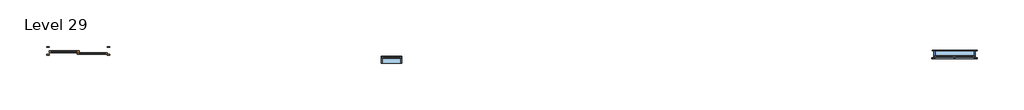
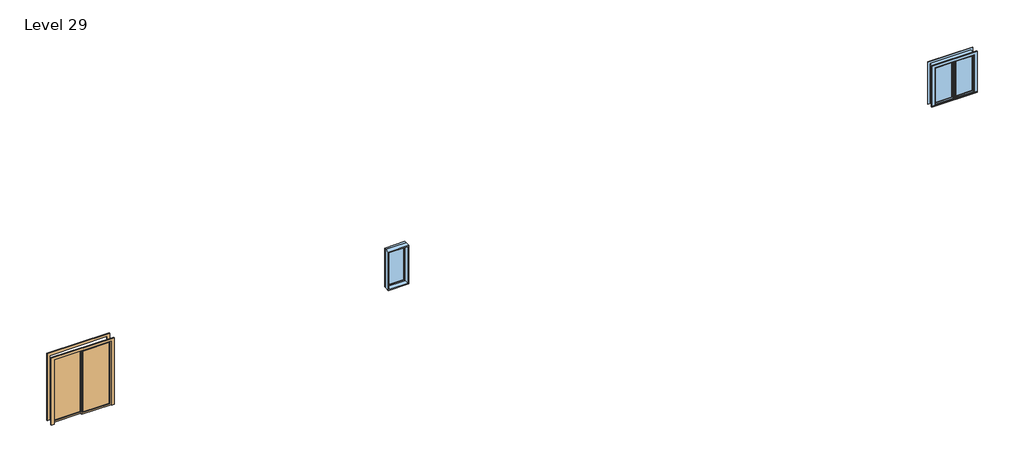
# One storey: 2 windows, 1 door.
"""IFC4 building model written with IfcOpenShell, lengths in millimetres."""

from ifc_helpers import new_model, si_unit, origin, place, context, project, spatial, transform, mapped, element, save
from components import door_076b30e0, window_0862ab64, window_80bd9af0

model = new_model("IFC4")

# Units and contexts
model_context = context("Model", 3, world=origin())
ifc_project = project(units=[si_unit("LENGTHUNIT", "METRE", prefix="MILLI")], contexts=[model_context])

# Site, building, storey
site = spatial("IfcSite", under=ifc_project)
building = spatial("IfcBuilding", under=site)
storey = spatial("IfcBuildingStorey", under=building, Name="Level 29", Elevation=49682.4)

# Door
placement = place(None, origin())
door_shape = door_076b30e0(model_context)
element("IfcDoor", 1, ObjectType="Door-Double-Sliding : 68\" x 80\"", at=placement, inside=storey, context=model_context, shape_type="MappedRepresentation", body=[
    mapped(door_shape, transform((-16064.585279, -12227.7237084, 49682.4), x_axis=(-1.0, 0.0, 0.0), y_axis=(0.0, -1.0, 0.0), z_axis=(0.0, 0.0, 1.0))),
])

# Windows
window_shape = window_0862ab64(model_context)
element("IfcWindow", 2, ObjectType="Casement Dbl with Trim : 48\" x 48\"", at=placement, inside=storey, context=model_context, shape_type="MappedRepresentation", body=[
    mapped(window_shape, transform((9924.3594464, -12437.2737084, 49682.4), x_axis=(-1.0, 0.0, 0.0), y_axis=(0.0, -1.0, 0.0), z_axis=(0.0, 0.0, 1.0))),
])
window_2_shape = window_80bd9af0(model_context)
element("IfcWindow", 3, ObjectType="Fixed : 24\" x 48\"", at=placement, inside=storey, context=model_context, shape_type="MappedRepresentation", body=[
    mapped(window_2_shape, transform((-6730.085279, -12617.2007309, 49682.4), x_axis=(1.0, 0.0, 0.0), y_axis=(0.0, 1.0, 0.0), z_axis=(0.0, 0.0, 1.0))),
])

save(model, "model.ifc")

# Revit data of these elements
# Type "Door-Double-Sliding : 68\" x 80\""
#   Type Mark = "10"
#   Construction Type Id = "opn-d45"
#   Assembly Code = "C1020"
#   Analytic Construction = "Wood frame, double glass door "
#   Thickness = 0' - 2"
#   Thermal Resistance (R) = 1.8150 (h·ft²·°F)/BTU
#   Heat Transfer Coefficient (U) = 0.5510 BTU/(h·ft²·°F)
#   Height = 6' - 8"
#   Rail Width = 0' - 2"
#   Stiles = 0' - 2"
#   Trim Projection Ext = 0' - 1"
#   Trim Projection Int = 0' - 1"
#   Trim Width = 0' - 3"
#   Width = 5' - 8"
#   Define Thermal Properties by = 1
#   Glazing = Glass
#   Panel Material = Wood - Birch - Solid Stained Light Low Gloss
#   Trim Material = Paint - Sienna
#   Visual Light Transmittance = 0
#   Solar Heat Gain Coefficient = 0
#   Function = (empty or 0)
#   Wall Closure = (empty or 0)
# Type "Casement Dbl with Trim : 48\" x 48\""
#   Type Mark = "34"
#   Construction Type Id = "GSP4R"
#   Assembly Code = "B2020100"
#   Analytic Construction = "1/8 in Pilkington single glazing"
#   Visual Light Transmittance = 0.9
#   Solar Heat Gain Coefficient = 0.78
#   Heat Transfer Coefficient (U) = 0.6496 BTU/(h·ft²·°F)
#   Height = 4' - 0"
#   Default Sill Height = 3' - 0"
#   Trim Projection - Ext. = 0' - 0 1/2"
#   Trim Projection - Int. = 0' - 0 3/4"
#   Trim Width - Exterior = 0' - 3 1/2"
#   Trim Width - Interior = 0' - 3 1/2"
#   Width = 4' - 0"
#   Window Inset = 0' - 0 3/4"
#   Define Thermal Properties by = 1
#   Glass Pane Material = Glass
#   Sash Material = Sash
#   Trim Exterior Material = Trim
#   Trim Interior Material = Trim
#   Wall Closure = (empty or 0)
# Type "Fixed : 24\" x 48\""
#   Type Mark = "2"
#   Construction Type Id = "GSP4R"
#   Assembly Code = "B2020100"
#   Analytic Construction = "1/8 in Pilkington single glazing"
#   Visual Light Transmittance = 0.9
#   Solar Heat Gain Coefficient = 0.78
#   Heat Transfer Coefficient (U) = 0.6496 BTU/(h·ft²·°F)
#   Height = 4' - 0"
#   Default Sill Height = 3' - 0"
#   Width = 2' - 0"
#   Window Inset = 0' - 0 3/4"
#   Define Thermal Properties by = 1
#   Glass Pane Material = Glass
#   Sash Material = Sash
#   Wall Closure = (empty or 0)
# Element 1 (IfcDoor, "Door-Double-Sliding : 68\" x 80\"")
#   Phase Created = New Construction
#   Materials on its faces: "Paint - Sienna", "Wood - Birch - Solid Stained Light Low Gloss", "Glass"
# Element 2 (IfcWindow, "Casement Dbl with Trim : 48\" x 48\"")
#   Mark = "2"
#   Phase Created = New Construction
#   Materials on its faces: "Sash", "Trim", "Glass"
# Element 3 (IfcWindow, "Fixed : 24\" x 48\"")
#   Mark = "70"
#   Phase Created = New Construction
#   Materials on its faces: "Sash", "Glass"
# Materials
#   "Glass": class "Glass", colour RGB 0 128 192, transparency 0.75, Description = "Soda Lime Glass", Cost = 0
#   "Wood - Birch - Solid Stained Light Low Gloss": class "Wood", colour RGB 210 159 95, transparency 0, Cost = 0
#   "Paint - Sienna": colour RGB 118 70 51, transparency 0, Cost = 0
#   "Sash": class "Wood", colour RGB 224 178 126, transparency 0
#   "Trim": class "Wood", colour RGB 224 178 126, transparency 0
